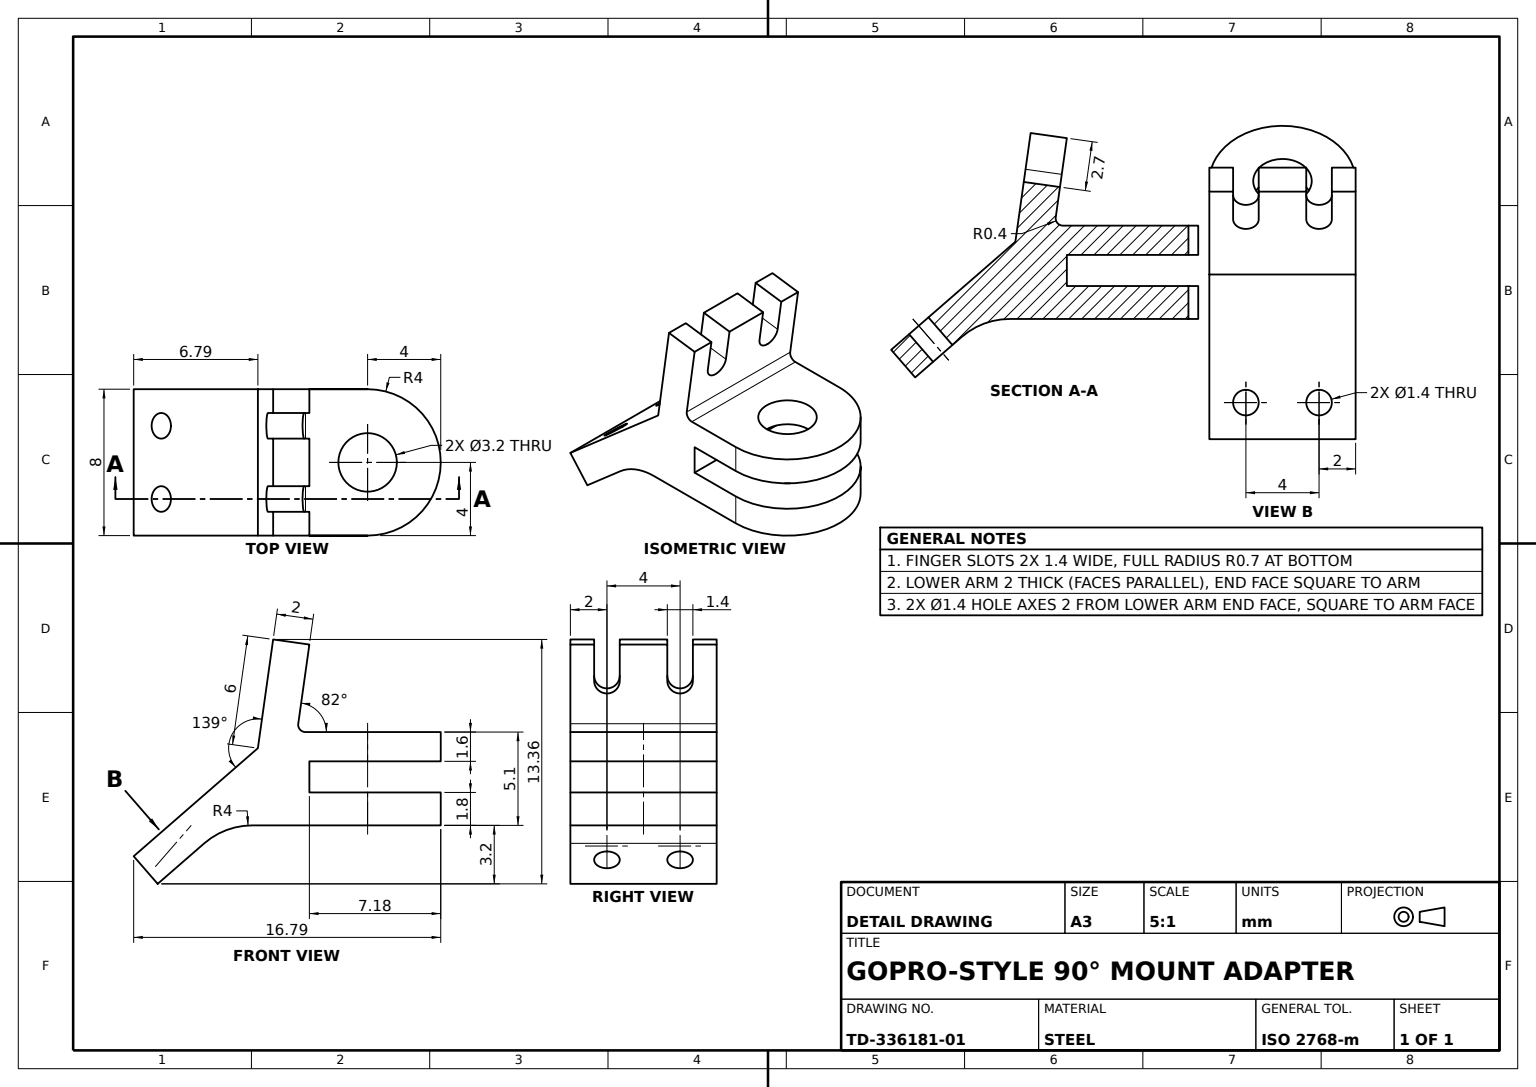
SolidWorks part; units mm, degrees
material "Plain Carbon Steel"
ref_plane "Front Plane" through (0, 0, 0) normal (0, 0, 1) x (1, 0, 0)
ref_plane "Top Plane" through (0, 0, 0) normal (0, 1, 0) x (1, 0, 0)
ref_plane "Right Plane" through (0, 0, 0) normal (1, 0, 0) x (0, 0, -1)
sketch "Base Arm Profile" plane through (0, 0, 0) normal (0, 0, 1) x (1, 0, 0)
  line L0 (0, 0) -> (-7.3567, -6.3951)
  line L1 (-7.3567, -6.3951) -> (-8.6689, -4.8857)
  line L2 (-8.6689, -4.8857) -> (-1.8765, 1.0188)
  line L3 (-1.8765, 1.0188) -> (-1.0414, 6.9604)
  line L5 (0.9391, 6.6821) -> (0, 0)
  line L13 (0.9391, 6.6821) -> (-1.0414, 6.9604)
  line L15 (0, 0) -> (11.9735, 0) construction
  dimension "D1" = 9
  dimension "D2" = 2
  dimension "D3" = 2
  dimension "D4" = 139
  dimension "D5" = 6
  dimension "D6" = 82
extrude "Base Arm 8mm" add sketch "Base Arm Profile" along normal mid plane 8
sketch "Finger Slots Profile" plane through (-1.9805, 0.2783, 0) normal (-0.9903, 0.1392, 0) x (0, 0, 1)
  line L0 (-2.7, 4.7478) -> (-2.7, 6.7478)
  line L1 (4, 6.7478) -> (-4, 6.7478) construction
  line L2 (-2.7, 6.7478) -> (-1.3, 6.7478)
  line L3 (-1.3, 6.7478) -> (-1.3, 4.7478)
  line L4 (0, 0) -> (0, 2.3131) construction
  line L5 (1.3, 6.7478) -> (1.3, 4.7478)
  line L6 (2.7, 6.7478) -> (1.3, 6.7478)
  line L7 (2.7, 4.7478) -> (2.7, 6.7478)
  arc A0 (-2.7, 4.7478) -> (-1.3, 4.7478) centre (-2, 4.7478) ccw
  arc A1 (2.7, 4.7478) -> (1.3, 4.7478) centre (2, 4.7478) cw
  dimension "D3" = 0.7
  dimension "D1" = 2
  dimension "D2" = 2
extrude "Finger Slots" cut sketch "Finger Slots Profile" against normal blind 8
sketch "Side Slot Profile" plane through (-1.3121, 1.5094, 0) normal (-0.6561, 0.7547, 0) x (0.7547, 0.6561, 0)
  line L0 (-9.7478, -4) -> (-9.7478, 4) construction
  line L1 (0, 0) -> (-6.8739, 0) construction
  circle A0 centre (-7.7478, -2) radius 0.7
  circle A1 centre (-7.7478, 2) radius 0.7
  dimension "D1" = 1.4
  dimension "D2" = 2
  dimension "D3" = 4
extrude "Side Slot" cut sketch "Side Slot Profile" against normal through all
sketch "Clevis Lug Profile" plane through (0, 0, 0) normal (0, 0, 1) x (1, 0, 0)
  line L0 (-3.6812, -3.2) -> (4.1235, -3.2)
  line L1 (-7.3567, -6.3951) -> (0, 0) construction
  line L2 (4.1235, -3.2) -> (4.1235, -1.4)
  line L3 (4.1235, -1.4) -> (0.9391, -1.4)
  line L4 (0.9391, -1.4) -> (0.9391, 0.3)
  line L5 (0.9391, 0.3) -> (4.1235, 0.3)
  line L6 (4.1235, 0.3) -> (4.1235, 1.9)
  line L7 (4.1235, 1.9) -> (0.267, 1.9)
  line L8 (0, 0) -> (0.9391, 6.6821) construction
  line L9 (-3.6812, -3.2) -> (0, 0)
  line L10 (0, 0) -> (0.267, 1.9)
  dimension "D1" = 5.1
  dimension "D2" = 1.6
  dimension "D3" = 1.9
  dimension "D4" = 3.3
  dimension "D5" = 6
extrude "Clevis Lug 8mm" add sketch "Clevis Lug Profile" along normal mid plane 8
fillet "Lug End Round R4" radius 4 1 edges at (-3.6812, -3.2, 0)
fillet "Edge Fillet R0.4" radius 0.4 1 edges at (0.267, 1.9, 0)
sketch "Lug Fill Boss Profile" plane through (0, -1.4, 0) normal (0, 1, 0) x (1, 0, 0)
  line L0 (4.1235, -4) -> (4.1235, 4) construction
  line L1 (4.1235, -4) -> (0.7272, -4) construction
  line L2 (4.1235, 4) -> (4.1235, -4)
  arc A0 (4.1235, 4) -> (4.1235, -4) centre (4.1235, 0) cw
extrude "Lug Fill Boss" add sketch "Lug Fill Boss Profile" against normal up to surface (1.8 mm away) up to face at (0.9689, -3.2, 0)
sketch "Lug Blend Boss Profile" plane through (0, 1.9, 0) normal (0, 1, 0) x (1, 0, 0)
  line L1 (4.1235, 4) -> (4.1235, -4)
  line L2 (4.1235, 4) -> (4.1235, -4)
  arc A1 (4.1235, -4) -> (4.1235, 4) centre (4.1235, 0) ccw
  arc A2 (4.1235, -4) -> (4.1235, 4) centre (4.1235, 0) ccw
  dimension "D1" = 0
extrude "Lug Blend Boss" add sketch "Lug Blend Boss Profile" against normal up to surface (1.6 mm away) up to face at (2.5313, 0.3, 0)
sketch "Pin Hole Profile" plane through (0, 1.9, 0) normal (0, 1, 0) x (1, 0, 0)
  circle A0 centre (4.1235, 0) radius 1.6
  arc A1 (4.1235, -4) -> (4.1235, 4) centre (4.1235, 0) ccw construction
  dimension "D1" = 3.2
extrude "Pin Hole Ø3.2" cut sketch "Pin Hole Profile" against normal through all
